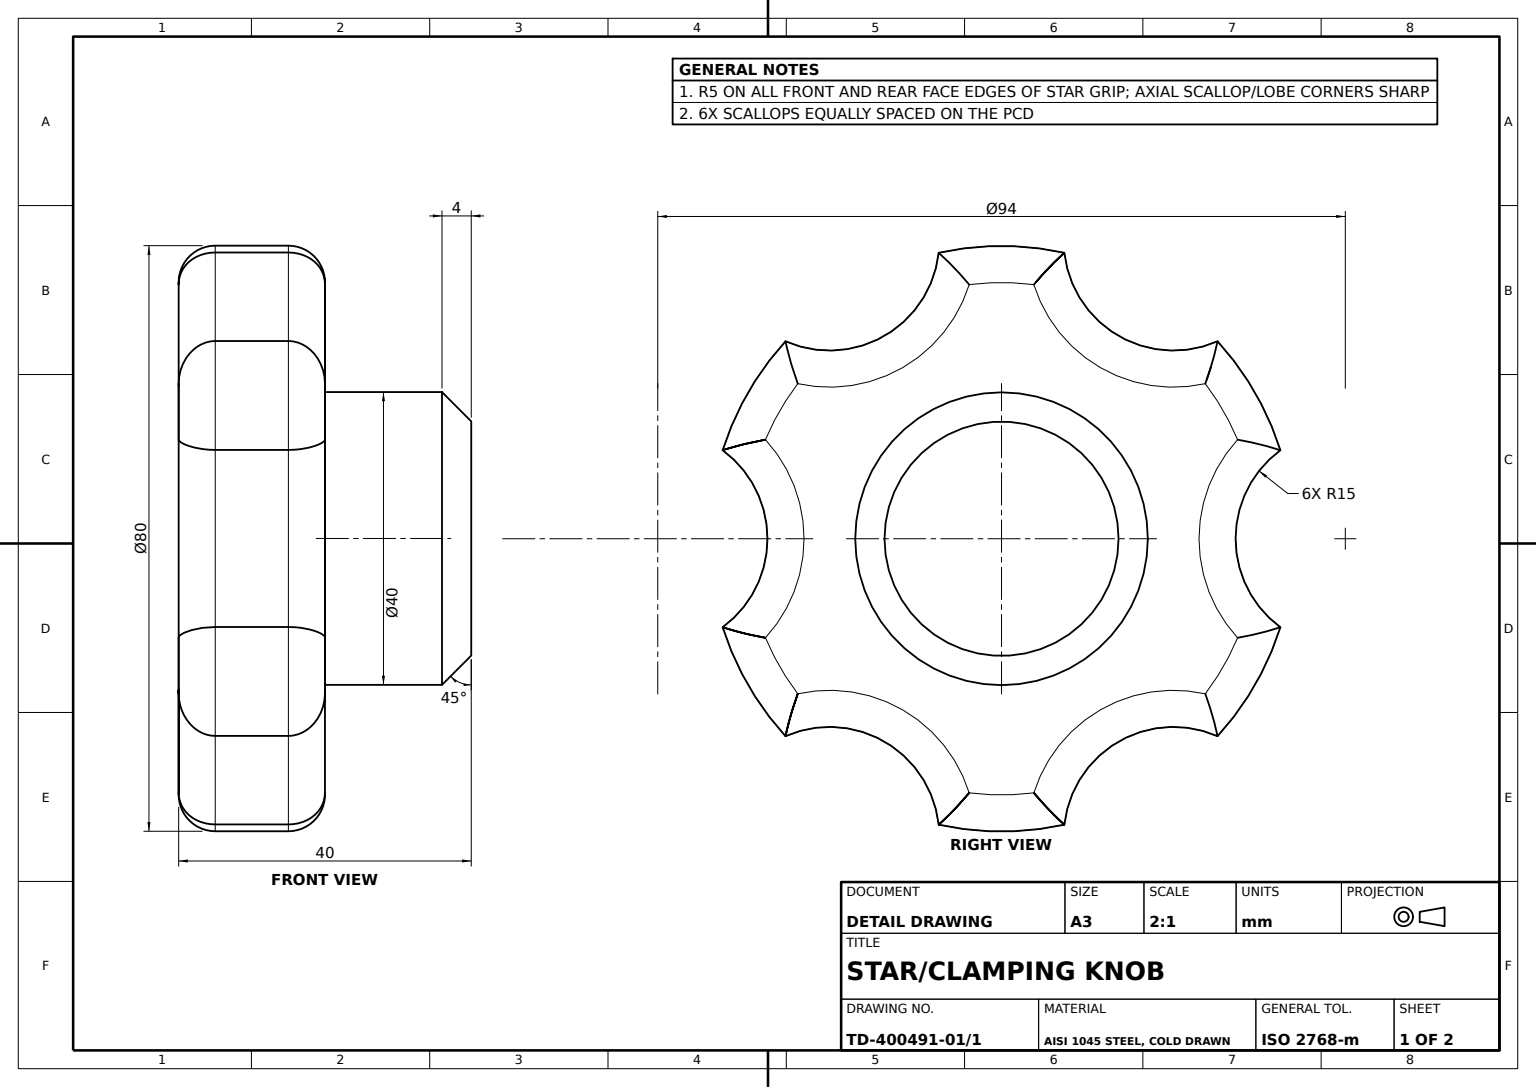
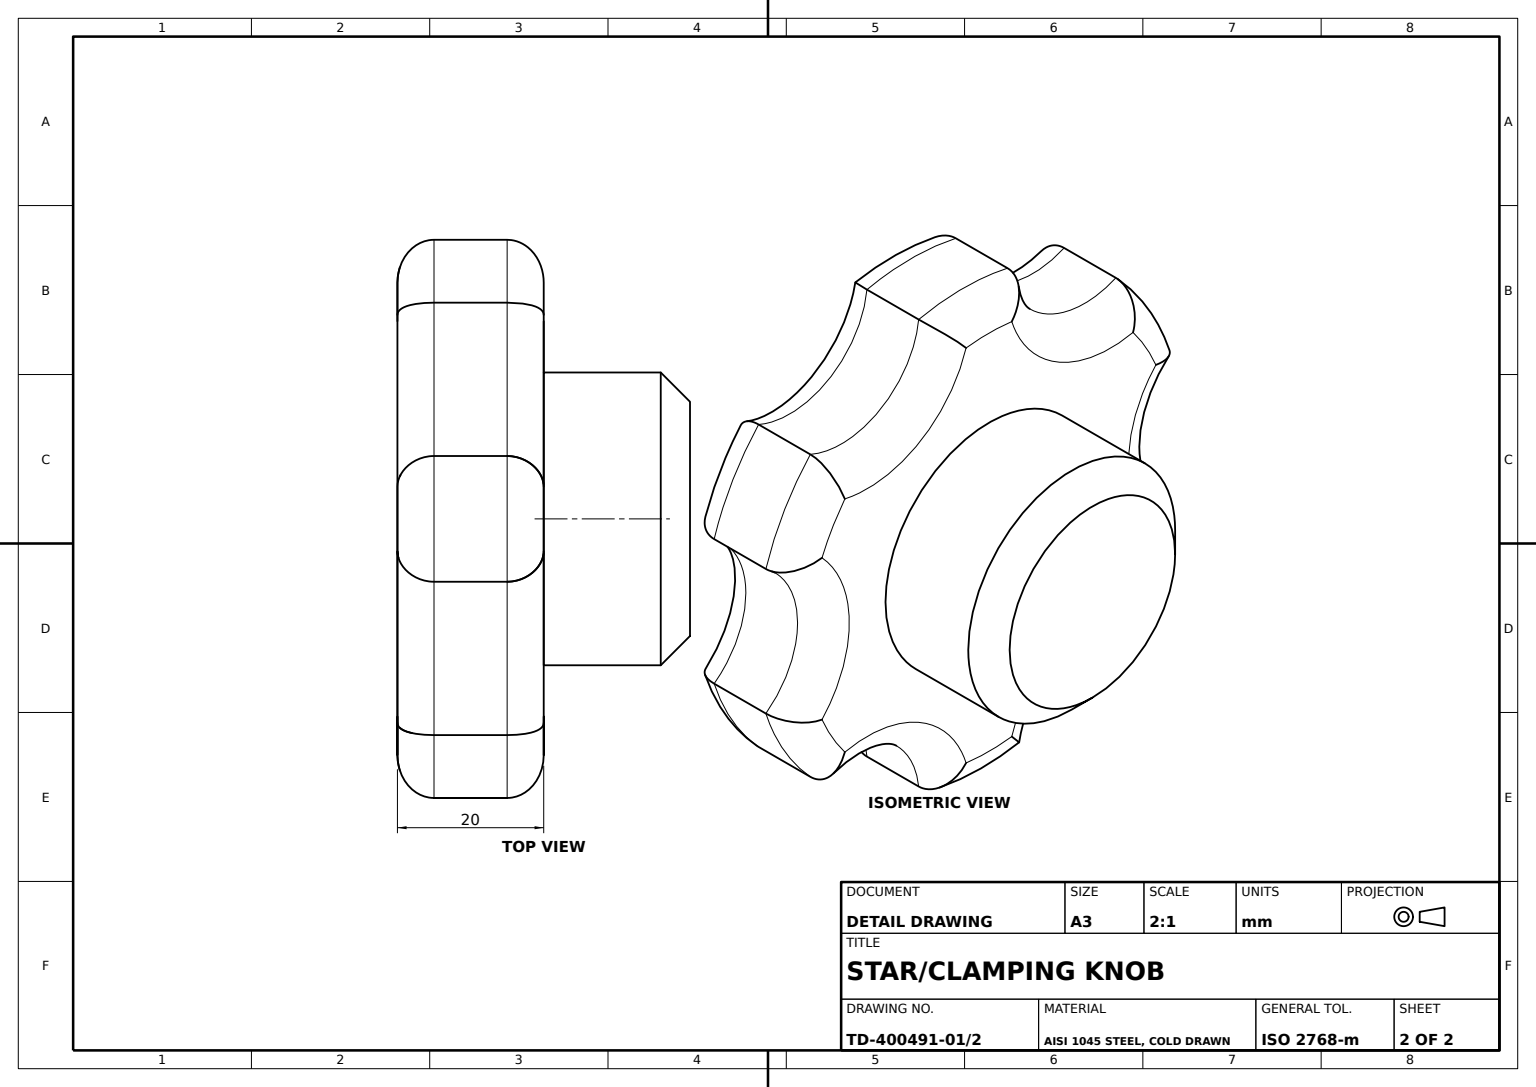
from build123d import *

# Parameters (mm, degrees)
STAR_GRIP_BODY_DEPTH      = 20
GRIP_EDGE_FILLET_R5_R     = 5
HUB_SKETCH_40_R           = 20
HUB_40_DEPTH              = 20
HUB_TOP_CHAMFER_4X45_SIZE = 4


with BuildPart() as part:
    # Star Profile Sketch → Star Grip Body (new body)
    with BuildSketch(Plane(origin=(0, 0, 0), x_dir=(1, 0, 0), z_dir=(0, 1, 0))):
        with BuildLine():
            ThreePointArc((-12.094692033, 38.127659574), (-20, 34.641016151), (-26.972175762, 29.538140339))
            ThreePointArc((-26.972175762, 29.538140339), (-27.712812921, 16), (-39.066867795, 8.589519236))
            ThreePointArc((-39.066867795, 8.589519236), (-40, 0), (-39.066867795, -8.589519236))
            ThreePointArc((-39.066867795, -8.589519236), (-27.712812921, -16), (-26.972175762, -29.538140339))
            ThreePointArc((-26.972175762, -29.538140339), (-20, -34.641016151), (-12.094692033, -38.127659574))
            ThreePointArc((-12.094692033, -38.127659574), (0, -32), (12.094692033, -38.127659574))
            ThreePointArc((12.094692033, -38.127659574), (20, -34.641016151), (26.972175762, -29.538140339))
            ThreePointArc((26.972175762, -29.538140339), (27.712812921, -16), (39.066867795, -8.589519236))
            ThreePointArc((39.066867795, -8.589519236), (40, 0), (39.066867795, 8.589519236))
            ThreePointArc((39.066867795, 8.589519236), (27.712812921, 16), (26.972175762, 29.538140339))
            ThreePointArc((26.972175762, 29.538140339), (20, 34.641016151), (12.094692033, 38.127659574))
            ThreePointArc((12.094692033, 38.127659574), (0, 32), (-12.094692033, 38.127659574))
        make_face()
    extrude(amount=STAR_GRIP_BODY_DEPTH)

    # Grip Edge Fillet R5
    grip_edge_fillet_r5_edges = [part.edges().sort_by_distance(p)[0] for p in [
        (27.712812921, 0, -16),
        (40, 0, 0),
        (-20, 20, -34.641016151),
        (27.712812921, 0, 16),
        (20, 0, 34.641016151),
        (0, 0, 32),
        (-20, 0, 34.641016151),
        (-27.712812921, 0, 16),
        (-40, 0, 0),
        (-27.712812921, 0, -16),
        (-20, 0, -34.641016151),
        (0, 0, -32),
        (20, 0, -34.641016151),
        (-27.712812921, 20, -16),
        (-40, 20, 0),
        (-27.712812921, 20, 16),
        (-20, 20, 34.641016151),
        (0, 20, 32),
        (20, 20, 34.641016151),
        (27.712812921, 20, 16),
        (40, 20, 0),
        (27.712812921, 20, -16),
        (20, 20, -34.641016151),
        (0, 20, -32),
    ]]
    fillet(grip_edge_fillet_r5_edges, radius=GRIP_EDGE_FILLET_R5_R)

    # Hub Sketch Ø40 → Hub Ø40 (add)
    with BuildSketch(Plane(origin=(0, 20, 0), x_dir=(1, 0, 0), z_dir=(0, 1, 0))):
        with Locations(Location((0, 0, 0), (0, 0, 270))):
            Circle(HUB_SKETCH_40_R)
    extrude(amount=HUB_40_DEPTH)

    # Hub Top Chamfer 4x45°
    hub_top_chamfer_4x45_edges = [part.edges().sort_by_distance(p)[0] for p in [
        (0, 40, -20),
    ]]
    chamfer(hub_top_chamfer_4x45_edges, length=HUB_TOP_CHAMFER_4X45_SIZE)


solid = part.part
